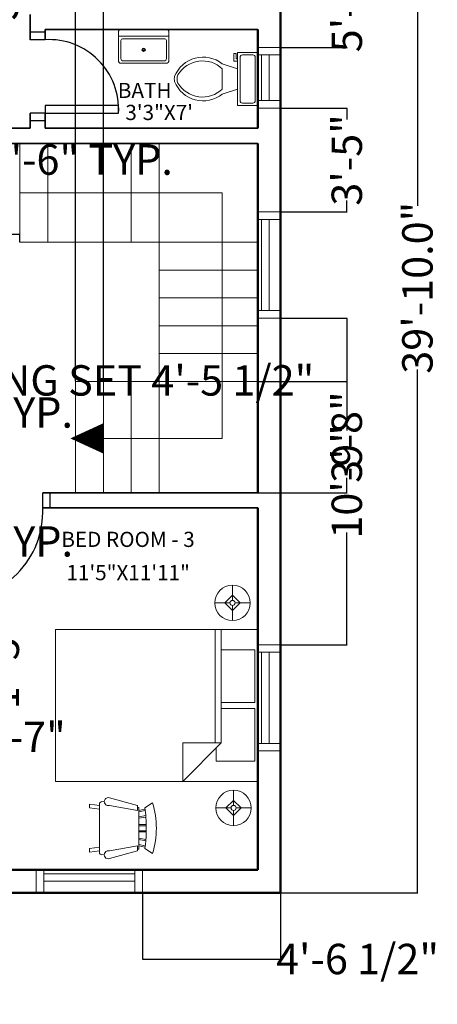
# Model space of a CAD drawing. Units: inches. Extents: x -52 to 472, y -40 to 644.
# Tile 5 of 6: x 250 to 415, y -40 to 349. Entities that reach past the tile are written whole.
import ezdxf

# ---------------------------------------------------------------- set-up
doc = ezdxf.new("R2010")
doc.units = ezdxf.units.IN
doc.header["$MEASUREMENT"] = 0
for name, color, linetype, lineweight in [('A-ANNO-DIMS', 7, 'Continuous', 13), ('A-ANNO-TEXT', 7, 'Continuous', 18), ('DOORS', 2, 'Continuous', 25), ('E-LIGHT', 30, 'Continuous', 13), ('FURNITURE', 6, 'Continuous', 13), ('INNER WALL', 1, 'Continuous', 35), ('OUTER WALL', 1, 'Continuous', 50), ('S-PLUM', 151, 'Continuous', 18), ('STAIRCASE', 3, 'Continuous', 18), ('VENTILATOR', 4, 'Continuous', 20), ('WINDOWS', 4, 'Continuous', 20)]:
    doc.layers.add(name, color=color, linetype=linetype, lineweight=lineweight)
doc.styles.get("Standard").update_dxf_attribs({"font": 'arial.ttf'})
doc.dimstyles.get("Standard").update_dxf_attribs({"dimtxt": 12, "dimasz": 0.18, "dimexe": 0.18, "dimexo": 0.0625, "dimgap": 0.09, "dimtad": 0, "dimdec": 1, "dimzin": 0, "dimdsep": 46, "dimlunit": 3, "dimtxsty": 'Standard', "dimcen": 0.09, "dimadec": 0, "dimazin": 0, "dimtfac": 1, "dimtdec": 1, "dimtofl": 0, "dimtmove": 0, "dimatfit": 3, "dimfxl": 1, "dimtolj": 1, "dimtzin": 0, "dimarcsym": 0})

# ---------------------------------------------------------------- blocks, each defined once
blk = doc.blocks.new('*D2')
at = {"layer": 'A-ANNO-DIMS', "color": 0, "lineweight": -2, "transparency": 16777216}
for p, q in [((353.19, 482.33), (407.42, 482.33)), ((407.24, 482.15), (407.24, 275.68)), ((407.24, 4.51), (407.24, 210.98)), ((353.19, 4.33), (407.42, 4.33))]:
    blk.add_line(p, q, dxfattribs=at)
at = {"layer": 'A-ANNO-DIMS', "color": 0, "transparency": 16777216}
for points in [[(407.21, 482.15), (407.27, 482.15), (407.24, 482.33)], [(407.21, 4.51), (407.27, 4.51), (407.24, 4.33)]]:
    blk.add_solid(points, dxfattribs=at)
at = {"layer": 'Defpoints', "color": 0, "transparency": 16777216}
for p in [(353.13, 482.33), (353.13, 4.33), (407.24, 4.33)]:
    blk.add_point(p, dxfattribs=at)
at = {"layer": 'A-ANNO-DIMS', "color": 0, "transparency": 16777216, "insert": (407.24, 243.33), "char_height": 12, "attachment_point": 5, "rotation": 90}
blk.add_mtext('\\A1;39\'-10.0"', dxfattribs=at)
blk = doc.blocks.new('Bed - Queen')
for p, q in [((0, -80.00003), (0, 0)), ((0, 0), (59.99999, 0)), ((59.99999, 0), (59.99999, -80.00003)), ((7.99999, -1.2), (28.79998, -1.2)), ((7.99999, -14.4), (7.99999, -1.2)), ((28.79998, -1.2), (28.79998, -14.4)), ((31.19999, -1.2), (51.99999, -1.2)), ((31.19999, -14.4), (31.19999, -1.2)), ((51.99999, -1.2), (51.99999, -16.4)), ((0, -14.4), (44.8, -14.4)), ((59.99999, -29.6), (44.8, -14.4)), ((44.8, -14.4), (44.8, -29.6)), ((44.8, -16.8), (0, -16.8)), ((51.99999, -16.4), (46.79936, -16.4)), ((44.8, -29.6), (59.99999, -29.6)), ((59.99999, -80.00003), (0, -80.00003))]:
    blk.add_line(p, q)
blk = doc.blocks.new('Toilet - top')
for p, q in [((9.5, -6), (9.5, -2)), ((-10, -8.5), (-8, -8.5)), ((-10, -9.5), (-10, -8.5)), ((-7, -9.5), (-10, -9.5)), ((-8, -8.5), (-8, -8)), ((-7, -8), (-7, -9.5)), ((-4, -8), (-6, -14)), ((4, -8), (6, -14)), ((4, -14), (-4, -14))]:
    blk.add_line(p, q)
blk.add_lwpolyline([(10.5, -8), (10.5, 0), (-10.5, 0), (-10.5, -8)], close=True)
for points in [[(-9.5, -2), (-9.5, -6)], [(8.5, -1), (-8.5, -1)], [(-8.5, -7), (8.5, -7)]]:
    blk.add_lwpolyline(points)
for centre, radius, start, end in [((-8.62, -1.88), 0.884, 81.8699, 188.1301), ((8.62, -1.88), 0.884, 351.8699, 98.1301), ((-8.62, -6.12), 0.884, 171.8699, 278.1301), ((8.62, -6.12), 0.884, 261.8699, 8.1301), ((3.52, -21.58), 12.17, 141.4691, 247.9714), ((4.2, -21.82), 11.33, 136.3677, 238.9468), ((-3.52, -21.58), 12.17, 292.0284, 38.5307), ((-4.2, -21.82), 11.33, 301.053, 43.6321), ((0, -27.88), 4, 245.7318, 294.2682), ((0, -29), 4, 254.8605, 285.1395)]:
    blk.add_arc(centre, radius, start, end)
blk = doc.blocks.new('Lamp - Table')
for p, q in [((0, 7), (0, 1)), ((-1, 0), (-7, 0)), ((0, 3), (-3, 0)), ((-3, 0), (0, -3)), ((3, 0), (0, 3)), ((0, -3), (3, 0)), ((1, 0), (7, 0)), ((0, -1), (0, -7))]:
    blk.add_line(p, q)
for radius in [7, 1]:
    blk.add_circle((0, 0), radius)
blk = doc.blocks.new('Sink-single - 30 in top')
blk.add_line((-15, -3.999996), (15, -3.999996))
for points in [[(-13.5, 0), (13.5, 0)], [(-15, -18.499996), (-15, -1.5)], [(-12.5, -5.499996), (12.5, -5.499996)], [(15, -1.5), (15, -18.499996)], [(-13.5, -17.499996), (-13.5, -6.499996)], [(13.5, -6.499996), (13.5, -17.499996)], [(13.5, -19.999996), (-13.5, -19.999996)], [(12.5, -18.499996), (-12.5, -18.499996)]]:
    blk.add_lwpolyline(points)
for radius in [1, 0.5]:
    blk.add_circle((0, -11.999996), radius)
for centre, radius, start, end in [((-13.5, -1.5), 1.5, 90, 180), ((-12.5, -6.499996), 1, 90, 180), ((12.5, -6.499996), 1, 0, 90), ((13.5, -1.5), 1.5, 0, 90), ((-12.5, -17.499996), 1, 180, 270), ((12.5, -17.499996), 1, 270, 0), ((-13.5, -18.499996), 1.5, 180, 270), ((13.5, -18.499996), 1.5, 270, 0)]:
    blk.add_arc(centre, radius, start, end)
blk = doc.blocks.new('*D15')
at = {"layer": 'A-ANNO-DIMS', "color": 0, "lineweight": -2, "transparency": 16777216}
for p, q in [((145.13, 258.39), (145.13, 264.49)), ((145.31, 264.31), (174.59, 264.31)), ((249.95, 264.31), (220.67, 264.31)), ((250.13, 261.39), (250.13, 264.49))]:
    blk.add_line(p, q, dxfattribs=at)
at = {"layer": 'A-ANNO-DIMS', "color": 0, "transparency": 16777216}
for points in [[(145.31, 264.34), (145.31, 264.28), (145.13, 264.31)], [(249.95, 264.34), (249.95, 264.28), (250.13, 264.31)]]:
    blk.add_solid(points, dxfattribs=at)
at = {"layer": 'Defpoints', "color": 0, "transparency": 16777216}
for p in [(250.13, 264.31), (250.13, 261.33), (145.13, 258.33)]:
    blk.add_point(p, dxfattribs=at)
at = {"layer": 'A-ANNO-DIMS', "color": 0, "transparency": 16777216, "insert": (197.63, 264.31), "char_height": 12, "attachment_point": 5}
blk.add_mtext('\\A1;8\'-9.0"', dxfattribs=at)
blk = doc.blocks.new('Chair - Rocking')
for p, q in [((-8, -4.5), (-10, -1.5)), ((8, -4.5), (10, -1.5)), ((-9, -7.5), (-12, -18.49999)), ((-7, -7.5), (-9, -7.5)), ((-9, -18.49999), (-7, -7.5)), ((-8.23428, -6.99939), (-8.3093, -7.47958)), ((-8.23041, -7), (8.23915, -7)), ((-7.5, -4.5), (-7, -7)), ((-6.5, -7), (-7.02225, -4.43)), ((-4.5, -7), (-4.96674, -4.19951)), ((-4, -7), (-4.40532, -4.16272)), ((-1.5, -4.05012), (-1.5, -7)), ((-1, -7), (-1, -4.05012)), ((1, -7), (1, -4.04655)), ((1.5, -4.05012), (1.5, -7)), ((4, -7), (4.40187, -4.18694)), ((4.5, -7), (4.96761, -4.19437)), ((6.5, -7), (7, -4.4057)), ((7.5, -4.5), (7, -7)), ((7, -7.5), (9, -7.5)), ((9, -18.49999), (7, -7.5)), ((8.31071, -7.48854), (8.23449, -7.00073)), ((9, -7.5), (12, -18.49999)), ((-10.36644, -20.64523), (-10.5, -21.49999)), ((-9, -22.49999), (-9.5, -26.49999)), ((0, -22.49999), (-9.5, -22.49999)), ((-8, -26.49999), (-7.5, -22.49999)), ((0, -22.49999), (9.5, -22.49999)), ((8, -26.49999), (7.5, -22.49999)), ((9, -22.49999), (9.5, -26.49999)), ((10.5, -21.49999), (10.3575, -20.58798)), ((-9.5, -26.49999), (-8, -26.49999)), ((9.5, -26.49999), (8, -26.49999))]:
    blk.add_line(p, q)
for centre, radius, start, end in [((0, -34.08333), 34.08333, 72.93847, 107.0615), ((0, -68.25004), 64.25, 93.92211, 97.15267), ((0, -68.25004), 64.25, 82.84733, 93.92211), ((-10.5, -18.99999), 1.58114, 161.5651, 18.43495), ((10.5, -18.99999), 1.58114, 161.5651, 18.43495), ((-9.5, -21.49999), 1, 180, 270), ((9.5, -21.49999), 1, 270, 0)]:
    blk.add_arc(centre, radius, start, end)
blk = doc.blocks.new('WIN-36IN')
for p, q in [((9, 42), (0, 42)), ((9, 39), (0, 39)), ((4.5, 3), (4.5, 39)), ((7.5, 3), (7.5, 39)), ((0, 3), (9, 3)), ((0, 0), (9, 0))]:
    blk.add_line(p, q)
blk = doc.blocks.new('WIN-36IN-SILL')
for p, q in [((0, 9), (0, 0)), ((3, 9), (3, 0)), ((39, 0), (39, 9)), ((42, 0), (42, 9)), ((3, 4.5), (39, 4.5)), ((3, 1.5), (39, 1.5)), ((3, 0), (39, 0))]:
    blk.add_line(p, q)
blk = doc.blocks.new('VENT-18IN')
for p, q in [((0, 9), (0, 0)), ((3, 9), (3, 0)), ((21, 0), (21, 9)), ((24, 0), (24, 9)), ((21, 7.5), (3, 7.5)), ((21, 4.5), (3, 4.5))]:
    blk.add_line(p, q)
blk = doc.blocks.new('*D32')
at = {"layer": 'A-ANNO-DIMS', "color": 0, "lineweight": -2, "transparency": 16777216}
for p, q in [((125.1, 196.98), (125.1, 193.87)), ((145.03, 196.98), (145.03, 193.87)), ((125.28, 194.05), (144.85, 194.05)), ((145.03, 194.05), (145.21, 194.05))]:
    blk.add_line(p, q, dxfattribs=at)
at = {"layer": 'A-ANNO-DIMS', "color": 0, "transparency": 16777216}
for points in [[(125.28, 194.08), (125.28, 194.02), (125.1, 194.05)], [(144.85, 194.08), (144.85, 194.02), (145.03, 194.05)]]:
    blk.add_solid(points, dxfattribs=at)
at = {"layer": 'Defpoints', "color": 0, "transparency": 16777216}
for p in [(125.1, 197.04), (145.03, 197.04), (145.03, 194.05)]:
    blk.add_point(p, dxfattribs=at)
at = {"layer": 'A-ANNO-DIMS', "color": 0, "transparency": 16777216, "insert": (209.09, 194.05), "char_height": 12, "attachment_point": 5}
blk.add_mtext('\\A1;BASIN 1\'-8" TYP.', dxfattribs=at)
blk = doc.blocks.new('*D41')
at = {"layer": 'A-ANNO-DIMS', "color": 0, "lineweight": -2, "transparency": 16777216}
for p, q in [((240.86, 79.26), (243.95, 79.26)), ((243.77, 79.26), (243.77, 79.44)), ((243.77, 62.21), (243.77, 79.08)), ((240.86, 62.03), (243.95, 62.03))]:
    blk.add_line(p, q, dxfattribs=at)
at = {"layer": 'A-ANNO-DIMS', "color": 0, "transparency": 16777216}
for points in [[(243.74, 79.08), (243.8, 79.08), (243.77, 79.26)], [(243.74, 62.21), (243.8, 62.21), (243.77, 62.03)]]:
    blk.add_solid(points, dxfattribs=at)
at = {"layer": 'Defpoints', "color": 0, "transparency": 16777216}
for p in [(240.8, 79.26), (243.77, 79.26), (240.8, 62.03)]:
    blk.add_point(p, dxfattribs=at)
at = {"layer": 'A-ANNO-DIMS', "color": 0, "transparency": 16777216, "insert": (243.77, 94.91), "char_height": 12, "attachment_point": 5, "rotation": 90}
blk.add_mtext('\\A1;1\'-5"', dxfattribs=at)
blk = doc.blocks.new('*D50')
at = {"layer": 'A-ANNO-DIMS', "color": 0, "lineweight": -2, "transparency": 16777216}
for p, q in [((237.19, 342.75), (243.68, 342.75)), ((243.5, 342.75), (243.5, 342.93)), ((243.5, 300.51), (243.5, 342.57)), ((237.19, 300.33), (243.68, 300.33))]:
    blk.add_line(p, q, dxfattribs=at)
at = {"layer": 'A-ANNO-DIMS', "color": 0, "transparency": 16777216}
for points in [[(243.47, 342.57), (243.53, 342.57), (243.5, 342.75)], [(243.47, 300.51), (243.53, 300.51), (243.5, 300.33)]]:
    blk.add_solid(points, dxfattribs=at)
at = {"layer": 'Defpoints', "color": 0, "transparency": 16777216}
for p in [(237.13, 342.75), (243.5, 342.75), (237.13, 300.33)]:
    blk.add_point(p, dxfattribs=at)
at = {"layer": 'A-ANNO-DIMS', "color": 0, "transparency": 16777216, "insert": (243.5, 454.09), "char_height": 12, "attachment_point": 5, "rotation": 90}
blk.add_mtext('\\A1;SINGLE DOOR 3\'-6 1/2" TYP.', dxfattribs=at)
blk = doc.blocks.new('*D51')
at = {"layer": 'A-ANNO-DIMS', "color": 0, "lineweight": -2, "transparency": 16777216}
for p, q in [((195.13, 300.27), (195.13, 293.79)), ((237.13, 300.27), (237.13, 293.79)), ((195.31, 293.97), (236.95, 293.97)), ((237.13, 293.97), (237.31, 293.97))]:
    blk.add_line(p, q, dxfattribs=at)
at = {"layer": 'A-ANNO-DIMS', "color": 0, "transparency": 16777216}
for points in [[(195.31, 294), (195.31, 293.94), (195.13, 293.97)], [(236.95, 294), (236.95, 293.94), (237.13, 293.97)]]:
    blk.add_solid(points, dxfattribs=at)
at = {"layer": 'Defpoints', "color": 0, "transparency": 16777216}
for p in [(195.13, 300.33), (237.13, 300.33), (237.13, 293.97)]:
    blk.add_point(p, dxfattribs=at)
at = {"layer": 'A-ANNO-DIMS', "color": 0, "transparency": 16777216, "insert": (273.97, 293.97), "char_height": 12, "attachment_point": 5}
blk.add_mtext('\\A1;3\'-6" TYP.', dxfattribs=at)
blk = doc.blocks.new('*D53')
at = {"layer": 'A-ANNO-DIMS', "color": 0, "lineweight": -2, "transparency": 16777216}
for p, q in [((130.13, 136.81), (130.13, 143.29)), ((130.31, 143.11), (169.37, 143.11)), ((169.55, 136.81), (169.55, 143.29)), ((169.55, 143.11), (169.73, 143.11))]:
    blk.add_line(p, q, dxfattribs=at)
at = {"layer": 'A-ANNO-DIMS', "color": 0, "transparency": 16777216}
for points in [[(130.31, 143.14), (130.31, 143.08), (130.13, 143.11)], [(169.37, 143.14), (169.37, 143.08), (169.55, 143.11)]]:
    blk.add_solid(points, dxfattribs=at)
at = {"layer": 'Defpoints', "color": 0, "transparency": 16777216}
for p in [(169.55, 143.11), (130.13, 136.75), (169.55, 136.75)]:
    blk.add_point(p, dxfattribs=at)
at = {"layer": 'A-ANNO-DIMS', "color": 0, "transparency": 16777216, "insert": (220.37, 143.11), "char_height": 12, "attachment_point": 5}
blk.add_mtext('\\A1;3\'-3 1/2" TYP.', dxfattribs=at)
blk = doc.blocks.new('*D54')
at = {"layer": 'A-ANNO-DIMS', "color": 0, "lineweight": -2, "transparency": 16777216}
for p, q in [((154.49, 214.67), (154.49, 206.54)), ((207.9, 214.67), (207.9, 206.54)), ((154.67, 206.72), (207.72, 206.72)), ((207.9, 206.72), (208.08, 206.72))]:
    blk.add_line(p, q, dxfattribs=at)
at = {"layer": 'A-ANNO-DIMS', "color": 0, "transparency": 16777216}
for points in [[(154.67, 206.75), (154.67, 206.69), (154.49, 206.72)], [(207.72, 206.75), (207.72, 206.69), (207.9, 206.72)]]:
    blk.add_solid(points, dxfattribs=at)
at = {"layer": 'Defpoints', "color": 0, "transparency": 16777216}
for p in [(154.49, 214.73), (207.9, 214.73), (207.9, 206.72)]:
    blk.add_point(p, dxfattribs=at)
at = {"layer": 'A-ANNO-DIMS', "color": 0, "transparency": 16777216, "insert": (288.1, 206.72), "char_height": 12, "attachment_point": 5}
blk.add_mtext('\\A1;DINING SET 4\'-5 1/2"', dxfattribs=at)
blk = doc.blocks.new('*D56')
at = {"layer": 'A-ANNO-DIMS', "color": 0, "lineweight": -2, "transparency": 16777216}
for p, q in [((115.19, 70.43), (115.19, 65.67)), ((146.16, 70.43), (146.16, 65.67)), ((115.37, 65.85), (145.98, 65.85)), ((146.16, 65.85), (146.34, 65.85))]:
    blk.add_line(p, q, dxfattribs=at)
at = {"layer": 'A-ANNO-DIMS', "color": 0, "transparency": 16777216}
for points in [[(115.37, 65.88), (115.37, 65.82), (115.19, 65.85)], [(145.98, 65.88), (145.98, 65.82), (146.16, 65.85)]]:
    blk.add_solid(points, dxfattribs=at)
at = {"layer": 'Defpoints', "color": 0, "transparency": 16777216}
for p in [(115.19, 70.49), (146.16, 70.49), (146.16, 65.85)]:
    blk.add_point(p, dxfattribs=at)
at = {"layer": 'A-ANNO-DIMS', "color": 0, "transparency": 16777216, "insert": (208.7, 65.85), "char_height": 12, "attachment_point": 5}
blk.add_mtext('\\A1;LOVESEAT 2\'-7"', dxfattribs=at)
blk = doc.blocks.new('*D70')
at = {"layer": 'A-ANNO-DIMS', "color": 0, "lineweight": -2, "transparency": 16777216}
for p, q in [((353.194987, 398.808713), (379.512487, 398.808713)), ((379.332487, 398.988713), (379.332487, 399.168713)), ((353.194987, 338.308713), (379.512487, 338.308713)), ((379.332487, 338.128713), (379.332487, 337.948713))]:
    blk.add_line(p, q, dxfattribs=at)
at = {"layer": 'A-ANNO-DIMS', "color": 0, "transparency": 16777216}
for points in [[(379.302487, 398.988713), (379.362487, 398.988713), (379.332487, 398.808713)], [(379.302487, 338.128713), (379.362487, 338.128713), (379.332487, 338.308713)]]:
    blk.add_solid(points, dxfattribs=at)
at = {"layer": 'Defpoints', "color": 0, "transparency": 16777216}
for p in [(353.132487, 398.808713), (353.132487, 338.308713), (379.332487, 338.308713)]:
    blk.add_point(p, dxfattribs=at)
at = {"layer": 'A-ANNO-DIMS', "color": 0, "transparency": 16777216, "insert": (379.332487, 368.558713), "char_height": 12, "attachment_point": 5, "rotation": 90}
blk.add_mtext('\\A1;5\'-0 1/2"', dxfattribs=at)
blk = doc.blocks.new('*D71')
at = {"layer": 'A-ANNO-DIMS', "color": 0, "lineweight": -2, "transparency": 16777216}
for p, q in [((353.19, 314.31), (379.51, 314.31)), ((379.33, 314.13), (379.33, 309.85)), ((379.33, 273.51), (379.33, 277.78)), ((353.19, 273.33), (379.51, 273.33))]:
    blk.add_line(p, q, dxfattribs=at)
at = {"layer": 'A-ANNO-DIMS', "color": 0, "transparency": 16777216}
for points in [[(379.3, 314.13), (379.36, 314.13), (379.33, 314.31)], [(379.3, 273.51), (379.36, 273.51), (379.33, 273.33)]]:
    blk.add_solid(points, dxfattribs=at)
at = {"layer": 'Defpoints', "color": 0, "transparency": 16777216}
for p in [(353.13, 314.31), (353.13, 273.33), (379.33, 273.33)]:
    blk.add_point(p, dxfattribs=at)
at = {"layer": 'A-ANNO-DIMS', "color": 0, "transparency": 16777216, "insert": (379.33, 293.82), "char_height": 12, "attachment_point": 5, "rotation": 90}
blk.add_mtext('\\A1;3\'-5"', dxfattribs=at)
blk = doc.blocks.new('*D72')
at = {"layer": 'A-ANNO-DIMS', "color": 0, "lineweight": -2, "transparency": 16777216}
for p, q in [((353.19, 231.33), (379.51, 231.33)), ((379.33, 231.15), (379.33, 186.96)), ((379.33, 102.49), (379.33, 146.68)), ((353.19, 102.31), (379.51, 102.31))]:
    blk.add_line(p, q, dxfattribs=at)
at = {"layer": 'A-ANNO-DIMS', "color": 0, "transparency": 16777216}
for points in [[(379.3, 231.15), (379.36, 231.15), (379.33, 231.33)], [(379.3, 102.49), (379.36, 102.49), (379.33, 102.31)]]:
    blk.add_solid(points, dxfattribs=at)
at = {"layer": 'Defpoints', "color": 0, "transparency": 16777216}
for p in [(353.13, 231.33), (353.13, 102.31), (379.33, 102.31)]:
    blk.add_point(p, dxfattribs=at)
at = {"layer": 'A-ANNO-DIMS', "color": 0, "transparency": 16777216, "insert": (379.33, 166.82), "char_height": 12, "attachment_point": 5, "rotation": 90}
blk.add_mtext('\\A1;10\'-9"', dxfattribs=at)
blk = doc.blocks.new('*D73')
at = {"layer": 'A-ANNO-DIMS', "color": 0, "lineweight": -2, "transparency": 16777216}
for p, q in [((298.57, 4.27), (298.57, -22.05)), ((353.13, 4.27), (353.13, -22.05)), ((298.75, -21.87), (352.95, -21.87)), ((353.13, -21.87), (353.31, -21.87))]:
    blk.add_line(p, q, dxfattribs=at)
at = {"layer": 'A-ANNO-DIMS', "color": 0, "transparency": 16777216}
for points in [[(298.75, -21.84), (298.75, -21.9), (298.57, -21.87)], [(352.95, -21.84), (352.95, -21.9), (353.13, -21.87)]]:
    blk.add_solid(points, dxfattribs=at)
at = {"layer": 'Defpoints', "color": 0, "transparency": 16777216}
for p in [(298.57, 4.33), (353.13, 4.33), (353.13, -21.87)]:
    blk.add_point(p, dxfattribs=at)
at = {"layer": 'A-ANNO-DIMS', "color": 0, "transparency": 16777216, "insert": (383.57, -21.87), "char_height": 12, "attachment_point": 5}
blk.add_mtext('\\A1;4\'-6 1/2"', dxfattribs=at)
blk = doc.blocks.new('*D78')
at = {"layer": 'A-ANNO-DIMS', "color": 0, "lineweight": -2, "transparency": 16777216}
for p, q in [((344.19, 206.33), (379.51, 206.33)), ((379.33, 206.15), (379.33, 200.36)), ((379.33, 162.51), (379.33, 168.29)), ((344.19, 162.33), (379.51, 162.33))]:
    blk.add_line(p, q, dxfattribs=at)
at = {"layer": 'A-ANNO-DIMS', "color": 0, "transparency": 16777216}
for points in [[(379.3, 206.15), (379.36, 206.15), (379.33, 206.33)], [(379.3, 162.51), (379.36, 162.51), (379.33, 162.33)]]:
    blk.add_solid(points, dxfattribs=at)
at = {"layer": 'Defpoints', "color": 0, "transparency": 16777216}
for p in [(344.13, 206.33), (344.13, 162.33), (379.33, 162.33)]:
    blk.add_point(p, dxfattribs=at)
at = {"layer": 'A-ANNO-DIMS', "color": 0, "transparency": 16777216, "insert": (379.33, 184.33), "char_height": 12, "attachment_point": 5, "rotation": 90}
blk.add_mtext('\\A1;3\'-8"', dxfattribs=at)
blk = doc.blocks.new('*D79')
at = {"layer": 'A-ANNO-DIMS', "color": 0, "lineweight": -2, "transparency": 16777216}
for p, q in [((272.13, 206.39), (272.13, 508.71)), ((272.31, 508.53), (282.95, 508.53)), ((283.13, 206.39), (283.13, 508.71)), ((283.13, 508.53), (283.31, 508.53))]:
    blk.add_line(p, q, dxfattribs=at)
at = {"layer": 'A-ANNO-DIMS', "color": 0, "transparency": 16777216}
for points in [[(272.31, 508.56), (272.31, 508.5), (272.13, 508.53)], [(282.95, 508.56), (282.95, 508.5), (283.13, 508.53)]]:
    blk.add_solid(points, dxfattribs=at)
at = {"layer": 'Defpoints', "color": 0, "transparency": 16777216}
for p in [(283.13, 508.53), (272.13, 206.33), (283.13, 206.33)]:
    blk.add_point(p, dxfattribs=at)
at = {"layer": 'A-ANNO-DIMS', "color": 0, "transparency": 16777216, "insert": (304.01, 508.53), "char_height": 12, "attachment_point": 5}
blk.add_mtext('\\A1;0\'-11"', dxfattribs=at)

msp = doc.modelspace()

# ---------------------------------------------------------------- linework, layer by layer
at = {"layer": 'DOORS'}
for p, q in [((260.13, 344.33), (254.13, 344.33)), ((260.13, 341.33), (254.13, 341.33)), ((260.13, 312.33), (254.13, 312.33)), ((260.13, 309.33), (254.13, 309.33)), ((259.13, 156.33), (259.13, 162.33)), ((262.13, 156.33), (262.13, 162.33))]:
    msp.add_line(p, q, dxfattribs=at)
msp.add_lwpolyline([(260.13, 312.33), (289.13, 312.33), (289.13, 315.33), (260.13, 315.33)], close=True, dxfattribs=at)
for centre, radius, start, end in [((261.63, 313.83), 27.54, 356.8779, 93.1221), ((224.55, 154.83), 34.62, 267.5165, 2.4828)]:
    msp.add_arc(centre, radius, start, end, dxfattribs=at)
at = {"layer": 'INNER WALL'}
for p, q in [((254.13, 341.33), (254.13, 351.33)), ((344.13, 345.33), (260.13, 345.33)), ((260.13, 341.33), (260.13, 345.33)), ((254.13, 306.33), (254.13, 312.33)), ((260.13, 306.33), (260.13, 312.33)), ((254.13, 306.33), (234.13, 306.33)), ((344.13, 306.33), (260.13, 306.33)), ((344.13, 300.33), (234.13, 300.33)), ((259.13, 162.33), (344.13, 162.33)), ((259.13, 156.33), (344.13, 156.33))]:
    msp.add_line(p, q, dxfattribs=at)
at = {"layer": 'OUTER WALL'}
for p, q in [((344.13, 306.33), (344.13, 345.33)), ((344.13, 162.33), (344.13, 300.33)), ((344.13, 13.33), (344.13, 156.33)), ((217.13, 13.33), (344.13, 13.33))]:
    msp.add_line(p, q, dxfattribs=at)
msp.add_lwpolyline([(208.13, 4.33), (353.13, 4.33), (353.13, 482.33), (23.13, 482.33), (23.13, 4.33), (136.13, 4.33)], dxfattribs=at)
at = {"layer": 'STAIRCASE'}
for p, q in [((250.13, 261.33), (250.13, 300.33)), ((261.13, 261.33), (261.13, 300.33)), ((272.13, 261.33), (272.13, 300.33)), ((283.13, 261.33), (283.13, 300.33)), ((294.13, 261.33), (294.13, 300.33)), ((305.13, 162.33), (305.13, 300.33)), ((344.13, 261.33), (250.13, 261.33)), ((344.13, 261.33), (250.13, 261.33)), ((344.13, 250.33), (305.13, 250.33)), ((344.13, 239.33), (305.13, 239.33)), ((344.13, 228.33), (305.13, 228.33)), ((344.13, 217.33), (305.13, 217.33)), ((344.13, 206.33), (272.13, 206.33)), ((272.13, 162.33), (272.13, 206.33)), ((283.13, 162.33), (283.13, 206.33)), ((294.13, 162.33), (294.13, 206.33))]:
    msp.add_line(p, q, dxfattribs=at)
msp.add_lwpolyline([(250.13, 280.83), (330.07, 280.83), (330.07, 183.81), (283.13, 183.81)], dxfattribs=at)
msp.add_lwpolyline([(283.13, 183.81, 12, 0, 0), (270.07, 183.81, 0, 0, 0)], format="xyseb", dxfattribs=at)
at = {"layer": 'VENTILATOR'}
for p, q in [((344.13, 335.31), (344.13, 317.31)), ((353.13, 317.31), (353.13, 335.31))]:
    msp.add_line(p, q, dxfattribs=at)

# ---------------------------------------------------------------- block references
at = {"layer": 'E-LIGHT'}
for p in [(334.15, 118.81), (334.57, 37.81)]:
    msp.add_blockref('Lamp - Table', p, dxfattribs=at)
at = {"layer": 'FURNITURE', "rotation": 270}
for name, p in [('Bed - Queen', (344.13, 108.31)), ('Chair - Rocking', (304.07, 29.81))]:
    msp.add_blockref(name, p, dxfattribs=at)
at = {"layer": 'S-PLUM', "xscale": 0.6644285423771328, "yscale": 0.6644285423771328, "zscale": 0.6644285423771328}
msp.add_blockref('Sink-single - 30 in top', (299.04, 345.33), dxfattribs=at)
at = {"layer": 'S-PLUM', "rotation": 270}
msp.add_blockref('Toilet - top', (344.13, 325.81), dxfattribs=at)
at = {"layer": 'VENTILATOR', "rotation": 90.0000000000004}
msp.add_blockref('VENT-18IN', (353.13, 314.31), dxfattribs=at)
at = {"layer": 'WINDOWS'}
for name, p, rotation in [('WIN-36IN', (353.13, 273.33), 180), ('WIN-36IN-SILL', (344.13, 102.31), 269.9999999999997), ('WIN-36IN', (298.57, 4.33), 90.00000000000017)]:
    msp.add_blockref(name, p, dxfattribs=dict(at, rotation=rotation))

# ---------------------------------------------------------------- texts
at = {"layer": 'A-ANNO-TEXT'}
for s, p in [('BATH', (288.83, 318.28)), ('3\'3"X7\'', (291.8, 309.59)), ('BED ROOM - 3', (266.51, 140.92)), ('11\'5"X11\'11"', (268.51, 127.78))]:
    msp.add_text(s, height=6, dxfattribs=at).set_placement(p)

# ---------------------------------------------------------------- dimensions: what is measured, and where the dimension line sits
at = {"layer": 'A-ANNO-DIMS'}
dim = msp.add_linear_dim(base=(243.5, 342.75), p1=(237.13, 300.33), p2=(237.13, 342.75), angle=90, text='SINGLE DOOR <> TYP.', dimstyle='Standard', override={"dimdec": 1, "dimlfac": 1, "dimrnd": 0, "dimzin": 1, "dimdsep": 46, "dimlunit": 4, "dimfrac": 2}, dxfattribs=at)
dim.commit()
dim.dimension.update_dxf_attribs({"geometry": '*D50', "text_midpoint": (243.5, 454.09)})
for base, p1, p2, override, picture, middle in [((283.13, 508.53), (272.13, 206.33), (283.13, 206.33), {"dimdec": 1, "dimlfac": 1, "dimrnd": 0, "dimzin": 1, "dimdsep": 46, "dimlunit": 4, "dimfrac": 2}, '*D79', (304.01, 508.53)), ((250.13, 264.31), (145.13, 258.33), (250.13, 261.33), {"dimclrd": 0, "dimclre": 0, "dimclrt": 0}, '*D15', (197.63, 264.31)), ((353.13, -21.87), (298.57, 4.33), (353.13, 4.33), {"dimdec": 1, "dimlfac": 1, "dimrnd": 0, "dimzin": 1, "dimdsep": 46, "dimlunit": 4, "dimfrac": 2}, '*D73', (383.57, -21.87))]:
    dim = msp.add_linear_dim(base=base, p1=p1, p2=p2, dimstyle='Standard', override=override, dxfattribs=at)
    dim.commit()
    dim.dimension.update_dxf_attribs({"geometry": picture, "text_midpoint": middle})
for base, p1, p2, override, picture, middle in [((407.24, 4.33), (353.13, 482.33), (353.13, 4.33), {"dimclrd": 0, "dimclre": 0, "dimclrt": 0}, '*D2', (407.24, 243.33)), ((379.33, 338.31), (353.13, 398.81), (353.13, 338.31), {"dimdec": 1, "dimlfac": 1, "dimrnd": 0, "dimzin": 1, "dimdsep": 46, "dimlunit": 4, "dimfrac": 2}, '*D70', (379.33, 368.56)), ((379.33, 273.33), (353.13, 314.31), (353.13, 273.33), {"dimdec": 1, "dimlfac": 1, "dimrnd": 0, "dimzin": 1, "dimdsep": 46, "dimlunit": 4, "dimfrac": 2}, '*D71', (379.33, 293.82)), ((379.33, 102.31), (353.13, 231.33), (353.13, 102.31), {"dimdec": 1, "dimlfac": 1, "dimrnd": 0, "dimzin": 1, "dimdsep": 46, "dimlunit": 4, "dimfrac": 2}, '*D72', (379.33, 166.82)), ((379.33, 162.33), (344.13, 206.33), (344.13, 162.33), {"dimdec": 1, "dimlfac": 1, "dimrnd": 0, "dimzin": 1, "dimdsep": 46, "dimlunit": 4, "dimfrac": 2}, '*D78', (379.33, 184.33)), ((243.77, 79.26), (240.8, 62.03), (240.8, 79.26), {"dimdec": 1, "dimlfac": 1, "dimrnd": 0, "dimzin": 1, "dimdsep": 46, "dimlunit": 4, "dimfrac": 2}, '*D41', (243.77, 94.91))]:
    dim = msp.add_linear_dim(base=base, p1=p1, p2=p2, angle=90, dimstyle='Standard', override=override, dxfattribs=at)
    dim.commit()
    dim.dimension.update_dxf_attribs({"geometry": picture, "text_midpoint": middle})
for base, p1, p2, text, picture, middle in [((237.13, 293.97), (195.13, 300.33), (237.13, 300.33), '<> TYP.', '*D51', (273.97, 293.97)), ((207.9, 206.72), (154.49, 214.73), (207.9, 214.73), 'DINING SET <>', '*D54', (288.1, 206.72)), ((145.03, 194.05), (125.1, 197.04), (145.03, 197.04), 'BASIN <> TYP.', '*D32', (209.09, 194.05)), ((169.55, 143.11), (130.13, 136.75), (169.55, 136.75), '<> TYP.', '*D53', (220.37, 143.11)), ((146.16, 65.85), (115.19, 70.49), (146.16, 70.49), 'LOVESEAT <>', '*D56', (208.7, 65.85))]:
    dim = msp.add_linear_dim(base=base, p1=p1, p2=p2, text=text, dimstyle='Standard', override={"dimdec": 1, "dimlfac": 1, "dimrnd": 0, "dimzin": 1, "dimdsep": 46, "dimlunit": 4, "dimfrac": 2}, dxfattribs=at)
    dim.commit()
    dim.dimension.update_dxf_attribs({"geometry": picture, "text_midpoint": middle})

doc.saveas('drawing.dxf')
